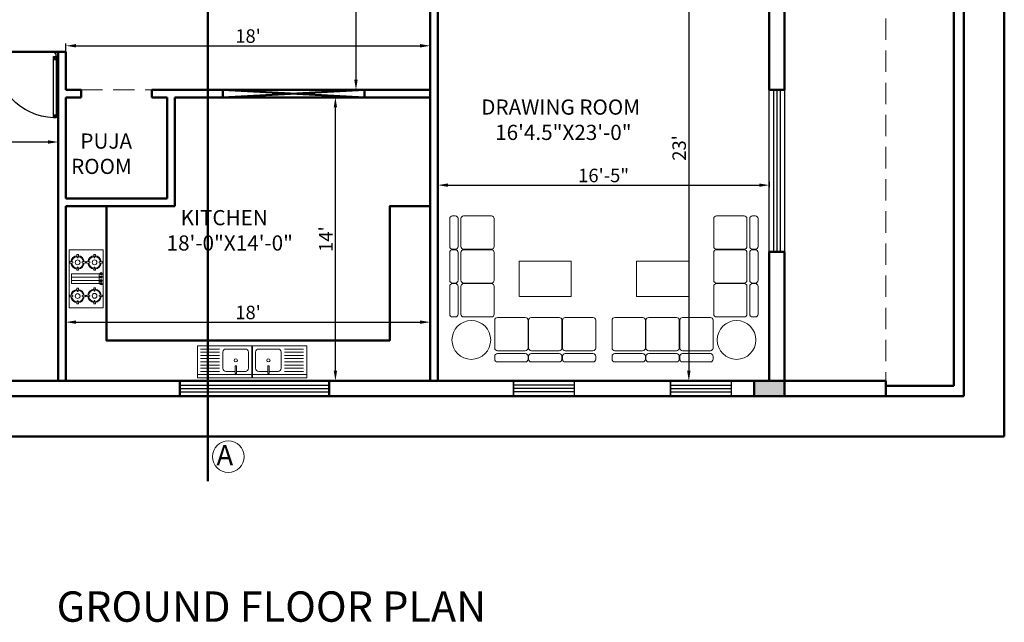
# Model space of a CAD drawing. Units: millimetres. Extents: x 1706 to 5913, y 156 to 1716.
# Tile 16 of 26: x 3489 to 4073, y 1031 to 1388. Entities that reach past the tile are written whole.
import ezdxf

# ---------------------------------------------------------------- set-up
doc = ezdxf.new("R2010")
doc.units = ezdxf.units.MM
doc.linetypes.add('DASHED', pattern=[19.05, 12.7, -6.35])
for name, color, linetype, lineweight in [('A-ANNO-DIMS', 2, 'Continuous', 18), ('A-ANNO-SYMB', 3, 'Continuous', 18), ('A-ANNO-TEXT', 7, 'Continuous', 18), ('A-AREA-IDEN', 3, 'Continuous', 18), ('A-COLS', 20, 'Continuous', 50), ('A-DOOR', 4, 'Continuous', 25), ('A-FLOR-OVHD', 9, 'DASHED', 18), ('A-FURN', 8, 'Continuous', 18), ('A-GLAZ', 150, 'Continuous', 25), ('A-WALL', 7, 'Continuous', 50)]:
    doc.layers.add(name, color=color, linetype=linetype, lineweight=lineweight)
doc.styles.get("Standard").update_dxf_attribs({"font": 'arial.ttf'})
doc.dimstyles.new('ISO-25', dxfattribs={"dimtxt": 8, "dimasz": 6, "dimexe": 1.25, "dimexo": 0.625, "dimtad": 1, "dimdec": 0, "dimlunit": 3, "dimtxsty": 'Standard', "dimcen": 2.5, "dimadec": 0, "dimazin": 0, "dimtfac": 1, "dimtdec": 0, "dimtmove": 0, "dimatfit": 3, "dimfxl": 1, "dimarcsym": 0})

# ---------------------------------------------------------------- blocks, each defined once
blk = doc.blocks.new('Puerta 01')
for p, q in [((-0.775, -0.026), (-0.737, -0.058)), ((-0.775, -0.058), (-0.737, -0.026)), ((-0.737, -0.058), (-0.737, -0.026)), ((-0.028, -0.058), (-0.066, -0.026)), ((-0.028, -0.026), (-0.066, -0.058)), ((-0.066, -0.058), (-0.066, -0.026))]:
    blk.add_line(p, q)
for points in [[(-0.028, 0), (-0.028, -0.026), (0.004, -0.026), (0.004, -0.036), (0.028, -0.036), (0.028, 0)], [(-0.028, -0.026), (-0.775, -0.026), (-0.775, -0.058), (-0.028, -0.058)], [(0.004, -0.774), (0.004, -0.764), (0.028, -0.764), (0.028, -0.8), (-0.028, -0.8), (-0.028, -0.774)]]:
    blk.add_lwpolyline(points, close=True)
blk.add_arc((-0.028, -0.026), 0.747, 182.4545, 270)
blk = doc.blocks.new('A$C57CF26DA')
for p, q in [((0, 0), (0, 420)), ((720, 420), (0, 420)), ((167, 413), (147, 413)), ((147, 413), (152, 373)), ((152, 373), (162, 373)), ((162, 373), (167, 413)), ((300, 391), (300, 49)), ((300, 391), (420, 391)), ((340, 391), (340, 49)), ((380, 391), (380, 49)), ((420, 391), (420, 49)), ((584, 413), (564, 413)), ((564, 413), (569, 373)), ((569, 373), (579, 373)), ((579, 373), (584, 413)), ((720, 0), (720, 420)), ((99, 320), (59, 325)), ((59, 325), (59, 305)), ((59, 305), (99, 310)), ((99, 310), (99, 320)), ((152, 257), (147, 217)), ((162, 257), (152, 257)), ((167, 217), (162, 257)), ((255, 325), (215, 320)), ((215, 320), (215, 310)), ((215, 310), (255, 305)), ((255, 305), (255, 325)), ((516, 320), (476, 325)), ((476, 325), (476, 305)), ((476, 305), (516, 310)), ((516, 310), (516, 320)), ((569, 257), (564, 217)), ((579, 257), (569, 257)), ((584, 217), (579, 257)), ((672, 325), (632, 320)), ((632, 320), (632, 310)), ((632, 310), (672, 305)), ((672, 305), (672, 325)), ((147, 217), (167, 217)), ((167, 203), (147, 203)), ((147, 203), (152, 163)), ((152, 163), (162, 163)), ((162, 163), (167, 203)), ((581, 203), (561, 203)), ((561, 203), (566, 163)), ((564, 217), (584, 217)), ((566, 163), (576, 163)), ((576, 163), (581, 203)), ((99, 110), (59, 115)), ((59, 115), (59, 95)), ((59, 95), (99, 100)), ((99, 100), (99, 110)), ((152, 47), (147, 7)), ((147, 7), (167, 7)), ((162, 47), (152, 47)), ((167, 7), (162, 47)), ((255, 115), (215, 110)), ((215, 110), (215, 100)), ((215, 100), (255, 95)), ((255, 95), (255, 115)), ((302, 39), (295, 39)), ((295, 39), (295, 11)), ((295, 11), (302, 11)), ((420, 49), (300, 49)), ((302, 11), (302, 39)), ((341, 39), (334, 39)), ((334, 39), (334, 11)), ((334, 11), (341, 11)), ((341, 11), (341, 39)), ((380, 11), (380, 39)), ((380, 39), (386, 39)), ((386, 11), (380, 11)), ((386, 39), (386, 11)), ((419, 11), (419, 39)), ((419, 39), (426, 39)), ((426, 11), (419, 11)), ((426, 39), (426, 11)), ((513, 110), (473, 115)), ((473, 115), (473, 95)), ((473, 95), (513, 100)), ((513, 100), (513, 110)), ((566, 47), (561, 7)), ((561, 7), (581, 7)), ((576, 47), (566, 47)), ((581, 7), (576, 47)), ((669, 115), (629, 110)), ((629, 110), (629, 100)), ((629, 100), (669, 95)), ((669, 95), (669, 115)), ((720, 0), (0, 0))]:
    blk.add_line(p, q)
for centre in [(157, 315), (574, 315), (157, 105), (571, 105)]:
    blk.add_circle(centre, 30)
for centre, radius, start, end in [((157, 315), 83, 95.5849, 174.4151), ((157, 315), 73, 95.3738, 174.6262), ((157, 315), 73, 5.3738, 84.6262), ((157, 315), 83, 5.5849, 84.4151), ((574, 315), 83, 95.5849, 174.4151), ((574, 315), 73, 95.3738, 174.6262), ((574, 315), 73, 5.3738, 84.6262), ((574, 315), 83, 5.5849, 84.4151), ((157, 315), 83, 185.5849, 264.4151), ((157, 315), 73, 185.3738, 264.6262), ((157, 315), 73, 275.3738, 354.6262), ((157, 315), 83, 275.5849, 354.4151), ((574, 315), 83, 185.5849, 264.4151), ((574, 315), 73, 185.3738, 264.6262), ((574, 315), 73, 275.3738, 354.6262), ((574, 315), 83, 275.5849, 354.4151), ((157, 105), 83, 95.5849, 174.4151), ((157, 105), 73, 95.3738, 174.6262), ((157, 105), 73, 5.3738, 84.6262), ((157, 105), 83, 5.5849, 84.4151), ((571, 105), 83, 95.5849, 174.4151), ((571, 105), 73, 95.3738, 174.6262), ((571, 105), 73, 5.3738, 84.6262), ((571, 105), 83, 5.5849, 84.4151), ((157, 105), 83, 185.5849, 264.4151), ((157, 105), 73, 185.3738, 264.6262), ((157, 105), 73, 275.3738, 354.6262), ((157, 105), 83, 275.5849, 354.4151), ((298, 25), 13.7, 104.4775, 255.5225), ((298, 25), 13.7, 284.4775, 75.5225), ((337, 25), 13.7, 104.4775, 255.5225), ((337, 25), 13.7, 284.4775, 75.5225), ((383, 25), 13.7, 104.4775, 255.5225), ((383, 25), 13.7, 284.4775, 75.5225), ((422, 25), 13.7, 104.4775, 255.5225), ((422, 25), 13.7, 284.4775, 75.5225), ((571, 105), 83, 185.5849, 264.4151), ((571, 105), 73, 185.3738, 264.6262), ((571, 105), 73, 275.3738, 354.6262), ((571, 105), 83, 275.5849, 354.4151)]:
    blk.add_arc(centre, radius, start, end)
blk = doc.blocks.new('A$C3404121D')
for p, q in [((0, 0), (0, 500)), ((0, 500), (850, 500)), ((850, 500), (850, 0)), ((0, 450), (850, 450)), ((50, 100), (50, 350)), ((100, 400), (240, 400)), ((240, 431), (240, 425)), ((260, 431), (240, 431)), ((240, 425), (240, 315)), ((240, 315), (260, 315)), ((260, 431), (260, 315)), ((260, 400), (400, 400)), ((450, 100), (450, 350)), ((502, 400), (801, 400)), ((502, 350), (801, 350)), ((502, 300), (801, 300)), ((502, 250), (801, 250)), ((502, 200), (801, 200)), ((850, 0), (0, 0)), ((400, 50), (100, 50)), ((502, 150), (801, 150)), ((502, 100), (801, 100)), ((801, 50), (502, 50))]:
    blk.add_line(p, q)
blk.add_circle((250, 228), 25)
for centre, start, end in [((100, 350), 90, 180), ((400, 350), 0, 90), ((100, 100), 180, 270), ((400, 100), 270, 0)]:
    blk.add_arc(centre, 50, start, end)
blk = doc.blocks.new('A$C753D6792')
at = {"linetype": 'ByBlock'}
for p, q in [((0, 2530), (0, 2580)), ((50, 2630), (550, 2630)), ((600, 2580), (600, 2530)), ((610, 2530), (610, 2580)), ((660, 2630), (1160, 2630)), ((1210, 2580), (1210, 2530)), ((1220, 2530), (1220, 2580)), ((1270, 2630), (1770, 2630)), ((1820, 2580), (1820, 2530)), ((0, 1880), (0, 2380)), ((550, 2480), (50, 2480)), ((550, 2430), (50, 2430)), ((600, 2380), (600, 1880)), ((610, 1880), (610, 2380)), ((1160, 2480), (660, 2480)), ((1160, 2430), (660, 2430)), ((1210, 2380), (1210, 1880)), ((1220, 1880), (1220, 2380)), ((1770, 2480), (1270, 2480)), ((1770, 2430), (1270, 2430)), ((1820, 1880), (1820, 2380)), ((50, 1830), (427, 1830)), ((387, 1830), (550, 1830)), ((660, 1830), (1037, 1830)), ((997, 1830), (1160, 1830)), ((1270, 1830), (1647, 1830)), ((1607, 1830), (1770, 1830)), ((1880, 1820), (2380, 1820)), ((2530, 1820), (2580, 1820)), ((1830, 1770), (1830, 1393)), ((2430, 1270), (2430, 1770)), ((2480, 1270), (2480, 1770)), ((2630, 1770), (2630, 1270)), ((442, 815), (442, 1455)), ((442, 1455), (1372, 1455)), ((1382, 1455), (1382, 815)), ((1830, 1433), (1830, 1270)), ((1830, 1160), (1830, 783)), ((2380, 1220), (1880, 1220)), ((1880, 1210), (2380, 1210)), ((2430, 660), (2430, 1160)), ((2480, 660), (2480, 1160)), ((2580, 1220), (2530, 1220)), ((2530, 1210), (2580, 1210)), ((2630, 1160), (2630, 660)), ((1382, 815), (442, 815)), ((1830, 823), (1830, 660)), ((1830, 550), (1830, 173)), ((2380, 610), (1880, 610)), ((1880, 600), (2380, 600)), ((2430, 50), (2430, 550)), ((2480, 50), (2480, 550)), ((2580, 610), (2530, 610)), ((2530, 600), (2580, 600)), ((2630, 550), (2630, 50)), ((1830, 213), (1830, 50)), ((2380, 0), (1880, 0)), ((2580, 0), (2530, 0))]:
    blk.add_line(p, q, dxfattribs=at)
blk.add_circle((2242, 2235), 349, dxfattribs=at)
for centre, start, end in [((50, 2580), 90, 180), ((50, 2530), 180, 270), ((550, 2580), 0, 90), ((550, 2580), 0, 90), ((550, 2530), 270, 0), ((550, 2530), 270, 0), ((660, 2580), 90, 180), ((660, 2530), 180, 270), ((1160, 2580), 0, 90), ((1160, 2580), 0, 90), ((1160, 2530), 270, 0), ((1160, 2530), 270, 0), ((1270, 2580), 90, 180), ((1270, 2530), 180, 270), ((1770, 2580), 0, 90), ((1770, 2580), 0, 90), ((1770, 2530), 270, 0), ((1770, 2530), 270, 0), ((50, 2380), 90, 180), ((550, 2380), 0, 90), ((550, 2380), 0, 90), ((660, 2380), 90, 180), ((1160, 2380), 0, 90), ((1160, 2380), 0, 90), ((1270, 2380), 90, 180), ((1770, 2380), 0, 90), ((1770, 2380), 0, 90), ((50, 1880), 180, 270), ((550, 1880), 270, 0), ((660, 1880), 180, 270), ((1160, 1880), 270, 0), ((1270, 1880), 180, 270), ((1770, 1880), 270, 0), ((1880, 1770), 90, 180), ((2380, 1770), 0, 90), ((2530, 1770), 90, 180), ((2580, 1770), 0, 90), ((1880, 1270), 180, 270), ((2380, 1270), 270, 0), ((2380, 1270), 270, 0), ((2530, 1270), 180, 270), ((2530, 1270), 180, 270), ((2580, 1270), 270, 0), ((2580, 1270), 270, 0), ((1880, 1160), 90, 180), ((2380, 1160), 0, 90), ((2530, 1160), 90, 180), ((2580, 1160), 0, 90), ((1880, 660), 180, 270), ((1880, 550), 90, 180), ((2380, 660), 270, 0), ((2380, 660), 270, 0), ((2380, 550), 0, 90), ((2530, 660), 180, 270), ((2530, 660), 180, 270), ((2530, 550), 90, 180), ((2580, 660), 270, 0), ((2580, 660), 270, 0), ((2580, 550), 0, 90), ((1880, 50), 180, 270), ((2380, 50), 270, 0), ((2380, 50), 270, 0), ((2530, 50), 180, 270), ((2530, 50), 180, 270), ((2580, 50), 270, 0), ((2580, 50), 270, 0)]:
    blk.add_arc(centre, 50, start, end, dxfattribs=at)
blk = doc.blocks.new('*D51')
at = {"layer": 'A-ANNO-DIMS', "color": 0, "lineweight": -2, "transparency": 16777216}
for p, q in [((3231.71, 1314.9), (3231.71, 1316.48)), ((3237.71, 1315.23), (3506.21, 1315.23)), ((3512.21, 1314.9), (3512.21, 1316.48))]:
    blk.add_line(p, q, dxfattribs=at)
at = {"layer": 'A-ANNO-DIMS', "color": 0, "transparency": 16777216}
for points in [[(3237.71, 1316.23), (3237.71, 1314.23), (3231.71, 1315.23)], [(3506.21, 1316.23), (3506.21, 1314.23), (3512.21, 1315.23)]]:
    blk.add_solid(points, dxfattribs=at)
at = {"layer": 'Defpoints', "color": 0, "transparency": 16777216}
for p in [(3231.71, 1314.27), (3512.21, 1315.23), (3512.21, 1314.27)]:
    blk.add_point(p, dxfattribs=at)
at = {"layer": 'A-ANNO-DIMS', "color": 0, "transparency": 16777216, "insert": (3371.96, 1319.94), "char_height": 8, "attachment_point": 5}
blk.add_mtext('23\'-5"', dxfattribs=at)
blk = doc.blocks.new('*D58')
at = {"layer": 'A-ANNO-DIMS', "color": 0, "lineweight": -2, "transparency": 16777216}
for p, q in [((3686.08, 1503.68), (3689.93, 1503.68)), ((3688.68, 1497.68), (3688.68, 1352.18)), ((3686.08, 1346.18), (3689.93, 1346.18))]:
    blk.add_line(p, q, dxfattribs=at)
at = {"layer": 'A-ANNO-DIMS', "color": 0, "transparency": 16777216}
for points in [[(3687.68, 1497.68), (3689.68, 1497.68), (3688.68, 1503.68)], [(3687.68, 1352.18), (3689.68, 1352.18), (3688.68, 1346.18)]]:
    blk.add_solid(points, dxfattribs=at)
at = {"layer": 'Defpoints', "color": 0, "transparency": 16777216}
for p in [(3685.46, 1503.68), (3685.46, 1346.18), (3688.68, 1346.18)]:
    blk.add_point(p, dxfattribs=at)
at = {"layer": 'A-ANNO-DIMS', "color": 0, "transparency": 16777216, "insert": (3683.97, 1424.93), "char_height": 8, "attachment_point": 5, "rotation": 90}
blk.add_mtext('13\'-2"', dxfattribs=at)
blk = doc.blocks.new('*D59')
at = {"layer": 'A-ANNO-DIMS', "color": 0, "lineweight": -2, "transparency": 16777216}
for p, q in [((3516.71, 1359.93), (3516.71, 1373.5)), ((3522.71, 1372.25), (3726.71, 1372.25)), ((3732.71, 1359.93), (3732.71, 1373.5))]:
    blk.add_line(p, q, dxfattribs=at)
at = {"layer": 'A-ANNO-DIMS', "color": 0, "transparency": 16777216}
for points in [[(3522.71, 1373.25), (3522.71, 1371.25), (3516.71, 1372.25)], [(3726.71, 1373.25), (3726.71, 1371.25), (3732.71, 1372.25)]]:
    blk.add_solid(points, dxfattribs=at)
at = {"layer": 'Defpoints', "color": 0, "transparency": 16777216}
for p in [(3732.71, 1372.25), (3516.71, 1359.3), (3732.71, 1359.3)]:
    blk.add_point(p, dxfattribs=at)
at = {"layer": 'A-ANNO-DIMS', "color": 0, "transparency": 16777216, "insert": (3624.71, 1376.96), "char_height": 8, "attachment_point": 5}
blk.add_mtext("18'", dxfattribs=at)
blk = doc.blocks.new('*D60')
at = {"layer": 'A-ANNO-DIMS', "color": 0, "lineweight": -2, "transparency": 16777216}
for p, q in [((3677.47, 1341.68), (3675.23, 1341.68)), ((3676.48, 1179.68), (3676.48, 1335.68)), ((3677.47, 1173.68), (3675.23, 1173.68))]:
    blk.add_line(p, q, dxfattribs=at)
at = {"layer": 'A-ANNO-DIMS', "color": 0, "transparency": 16777216}
for points in [[(3675.48, 1335.68), (3677.48, 1335.68), (3676.48, 1341.68)], [(3675.48, 1179.68), (3677.48, 1179.68), (3676.48, 1173.68)]]:
    blk.add_solid(points, dxfattribs=at)
at = {"layer": 'Defpoints', "color": 0, "transparency": 16777216}
for p in [(3676.48, 1341.68), (3678.09, 1341.68), (3678.09, 1173.68)]:
    blk.add_point(p, dxfattribs=at)
at = {"layer": 'A-ANNO-DIMS', "color": 0, "transparency": 16777216, "insert": (3671.84, 1257.68), "char_height": 8, "attachment_point": 5, "rotation": 90}
blk.add_mtext("14'", dxfattribs=at)
blk = doc.blocks.new('*D61')
at = {"layer": 'A-ANNO-DIMS', "color": 0, "lineweight": -2, "transparency": 16777216}
for p, q in [((3516.71, 1201.14), (3516.71, 1209.73)), ((3522.71, 1208.48), (3726.71, 1208.48)), ((3732.71, 1201.14), (3732.71, 1209.73))]:
    blk.add_line(p, q, dxfattribs=at)
at = {"layer": 'A-ANNO-DIMS', "color": 0, "transparency": 16777216}
for points in [[(3522.71, 1209.48), (3522.71, 1207.48), (3516.71, 1208.48)], [(3726.71, 1209.48), (3726.71, 1207.48), (3732.71, 1208.48)]]:
    blk.add_solid(points, dxfattribs=at)
at = {"layer": 'Defpoints', "color": 0, "transparency": 16777216}
for p in [(3732.71, 1208.48), (3516.71, 1200.51), (3732.71, 1200.51)]:
    blk.add_point(p, dxfattribs=at)
at = {"layer": 'A-ANNO-DIMS', "color": 0, "transparency": 16777216, "insert": (3624.71, 1213.19), "char_height": 8, "attachment_point": 5}
blk.add_mtext("18'", dxfattribs=at)
blk = doc.blocks.new('*D62')
at = {"layer": 'A-ANNO-DIMS', "color": 0, "lineweight": -2, "transparency": 16777216}
for p, q in [((3882.51, 1449.68), (3887.24, 1449.68)), ((3885.99, 1443.68), (3885.99, 1179.68)), ((3882.51, 1173.68), (3887.24, 1173.68))]:
    blk.add_line(p, q, dxfattribs=at)
at = {"layer": 'A-ANNO-DIMS', "color": 0, "transparency": 16777216}
for points in [[(3884.99, 1443.68), (3886.99, 1443.68), (3885.99, 1449.68)], [(3884.99, 1179.68), (3886.99, 1179.68), (3885.99, 1173.68)]]:
    blk.add_solid(points, dxfattribs=at)
at = {"layer": 'Defpoints', "color": 0, "transparency": 16777216}
for p in [(3881.89, 1449.68), (3881.89, 1173.68), (3885.99, 1173.68)]:
    blk.add_point(p, dxfattribs=at)
at = {"layer": 'A-ANNO-DIMS', "color": 0, "transparency": 16777216, "insert": (3881.28, 1311.68), "char_height": 8, "attachment_point": 5, "rotation": 90}
blk.add_mtext("23'", dxfattribs=at)
blk = doc.blocks.new('*D63')
at = {"layer": 'A-ANNO-DIMS', "color": 0, "lineweight": -2, "transparency": 16777216}
for p, q in [((3737.21, 1291.56), (3737.21, 1288.41)), ((3933.71, 1291.56), (3933.71, 1288.41)), ((3743.21, 1289.66), (3927.71, 1289.66))]:
    blk.add_line(p, q, dxfattribs=at)
at = {"layer": 'A-ANNO-DIMS', "color": 0, "transparency": 16777216}
for points in [[(3743.21, 1290.66), (3743.21, 1288.66), (3737.21, 1289.66)], [(3927.71, 1290.66), (3927.71, 1288.66), (3933.71, 1289.66)]]:
    blk.add_solid(points, dxfattribs=at)
at = {"layer": 'Defpoints', "color": 0, "transparency": 16777216}
for p in [(3737.21, 1292.18), (3933.71, 1292.18), (3933.71, 1289.66)]:
    blk.add_point(p, dxfattribs=at)
at = {"layer": 'A-ANNO-DIMS', "color": 0, "transparency": 16777216, "insert": (3835.46, 1294.37), "char_height": 8, "attachment_point": 5}
blk.add_mtext('16\'-5"', dxfattribs=at)

msp = doc.modelspace()

# ---------------------------------------------------------------- hatches: boundary and pattern name
at = {"layer": 'A-COLS'}
h = msp.add_hatch(color=256, dxfattribs=at)
h.dxf.hatch_style = 1
h.paths.add_polyline_path([(3942.71, 1173.68), (3924.71, 1173.68), (3924.71, 1164.68), (3942.71, 1164.68)])

# ---------------------------------------------------------------- linework, layer by layer
at = {"layer": 'A-ANNO-SYMB'}
msp.add_circle((3613.03, 1128.74), 9.38, dxfattribs=at)
at = {"layer": 'A-COLS'}
msp.add_lwpolyline([(3942.93, 1173.68), (3924.71, 1173.68), (3924.71, 1164.68), (3942.71, 1164.68), (3942.71, 1173.68)], dxfattribs=at)
at = {"layer": 'A-FLOR-OVHD'}
for p, q in [((4002.71, 1655.18), (4002.71, 1173.68)), ((3525.71, 1346.18), (3567.71, 1346.18))]:
    msp.add_line(p, q, dxfattribs=at)
at = {"layer": 'A-GLAZ'}
for p, q in [((3936.21, 1346.18), (3936.21, 1250.18)), ((3938.21, 1346.18), (3938.21, 1250.18)), ((3940.21, 1346.18), (3940.21, 1250.18)), ((3782.07, 1173.68), (3782.07, 1164.68)), ((3818.07, 1173.68), (3818.07, 1164.68)), ((3875.07, 1173.68), (3875.07, 1164.68)), ((3911.07, 1173.68), (3911.07, 1164.68)), ((3584.21, 1171.18), (3672.71, 1171.18)), ((3584.21, 1169.18), (3672.71, 1169.18)), ((3818.07, 1171.18), (3782.07, 1171.18)), ((3818.07, 1169.18), (3782.07, 1169.18)), ((3875.07, 1171.18), (3911.07, 1171.18)), ((3875.07, 1169.18), (3911.07, 1169.18)), ((3584.21, 1167.18), (3672.71, 1167.18)), ((3818.07, 1167.18), (3782.07, 1167.18)), ((3875.07, 1167.18), (3911.07, 1167.18))]:
    msp.add_line(p, q, dxfattribs=at)
for points in [[(3933.71, 1346.18), (3942.71, 1346.18), (3942.71, 1250.18), (3933.71, 1250.18)], [(3584.21, 1173.68), (3672.71, 1173.68), (3672.71, 1164.68), (3584.21, 1164.68)], [(3782.07, 1173.68), (3818.07, 1173.68), (3818.07, 1164.68), (3782.07, 1164.68)], [(3875.07, 1173.68), (3911.07, 1173.68), (3911.07, 1164.68), (3875.07, 1164.68)]]:
    msp.add_lwpolyline(points, close=True, dxfattribs=at)
at = {"layer": 'A-WALL'}
for p, q in [((3600.83, 1703), (3600.83, 1114.32)), ((4049, 1664.18), (4049, 1164.68)), ((4073, 1664.18), (4073, 1140.68)), ((4043, 1658.18), (4043, 1170.68)), ((3732.71, 1410.68), (3732.71, 1173.68)), ((3737.21, 1410.68), (3737.21, 1173.68)), ((3933.71, 1403.18), (3933.71, 1346.18)), ((3942.71, 1403.18), (3942.71, 1346.18)), ((3473.21, 1368.68), (3512.21, 1368.68)), ((3512.21, 1368.68), (3516.71, 1368.68)), ((3512.21, 1368.68), (3512.21, 1173.68)), ((3516.71, 1368.68), (3516.71, 1346.18)), ((3516.71, 1346.18), (3525.71, 1346.18)), ((3525.71, 1346.18), (3525.71, 1341.68)), ((3567.71, 1346.18), (3567.71, 1341.68)), ((3567.71, 1346.18), (3609.71, 1346.18)), ((3609.71, 1346.18), (3609.71, 1341.68)), ((3693.71, 1346.18), (3609.71, 1341.68)), ((3609.71, 1346.18), (3693.71, 1341.68)), ((3693.71, 1346.18), (3693.71, 1341.68)), ((3693.71, 1346.18), (3732.71, 1346.18)), ((3942.71, 1346.18), (3933.71, 1346.18)), ((3516.71, 1341.68), (3525.71, 1341.68)), ((3516.71, 1341.68), (3516.71, 1281.68)), ((3567.71, 1341.68), (3576.71, 1341.68)), ((3576.71, 1341.68), (3576.71, 1281.68)), ((3581.21, 1341.68), (3581.21, 1277.18)), ((3581.21, 1341.68), (3609.71, 1341.68)), ((3693.71, 1341.68), (3732.71, 1341.68)), ((3516.71, 1281.68), (3576.71, 1281.68)), ((3516.71, 1277.18), (3581.21, 1277.18)), ((3516.71, 1277.18), (3516.71, 1173.68)), ((3942.71, 1250.18), (3933.71, 1250.18)), ((3933.71, 1250.18), (3933.71, 1173.68)), ((3942.71, 1250.18), (3942.71, 1173.68)), ((3207.71, 1173.68), (4002.71, 1173.68)), ((3584.21, 1173.68), (3584.21, 1164.68)), ((3672.71, 1173.68), (3672.71, 1164.68)), ((3942.71, 1173.68), (3942.71, 1164.68)), ((3942.71, 1164.68), (3942.71, 1173.68)), ((4002.71, 1173.68), (4002.71, 1164.68)), ((4043, 1170.68), (4002.71, 1170.68)), ((3203.21, 1164.68), (4002.71, 1164.68)), ((4049, 1164.68), (4002.71, 1164.68)), ((3177.71, 1140.68), (4073, 1140.68))]:
    msp.add_line(p, q, dxfattribs=at)
msp.add_lwpolyline([(3609.71, 1346.18), (3693.71, 1346.18), (3693.71, 1341.68), (3609.71, 1341.68)], close=True, dxfattribs=at)
msp.add_lwpolyline([(3540.71, 1277.18), (3540.71, 1197.68), (3708.71, 1197.68), (3708.71, 1277.18), (3732.71, 1277.18)], dxfattribs=at)

# ---------------------------------------------------------------- block references
at = {"layer": 'A-DOOR', "extrusion": (0, 0, -1), "xscale": 48.75000000000294, "yscale": 48.75000000000294, "zscale": -48.75000000000287, "rotation": 89.99999999879581}
msp.add_blockref('Puerta 01', (-3512.21, 1367.32), dxfattribs=at)
at = {"layer": 'A-FURN'}
for name, p, xscale, yscale, zscale, rotation in [('A$C753D6792', (3830.82, 1271.46), 0.0329035460231199, 0.0329035460231199, 0.0329035460231199, 180), ('A$C753D6792', (3840.51, 1271.46), -0.0329035460231199, 0.0329035460231199, 0.0329035460231199, 180), ('A$C57CF26DA', (3538.75, 1251.41), -0.0478777176975714, 0.0478777176975714, 0.0478777176975714, 90), ('A$C3404121D', (3626.89, 1194.45), 0.0378984485580132, 0.0378984485580132, 0.0378984485580132, 180), ('A$C3404121D', (3627.3, 1194.45), -0.0378984485580132, 0.0378984485580132, 0.0378984485580132, 180)]:
    msp.add_blockref(name, p, dxfattribs=dict(at, xscale=xscale, yscale=yscale, zscale=zscale, rotation=rotation))

# ---------------------------------------------------------------- texts
at = {"layer": 'A-ANNO-SYMB', "insert": (3602.29, 1135.61), "char_height": 12, "attachment_point": 1}
msp.add_mtext_dynamic_manual_height_columns(' A', width=23.3743, gutter_width=12.5, heights=[0], dxfattribs=at)
at = {"layer": 'A-ANNO-TEXT', "insert": (3511.24, 1048.93), "char_height": 18, "attachment_point": 1}
msp.add_mtext_dynamic_manual_height_columns('GROUND FLOOR PLAN', width=352.5721, gutter_width=12.5, heights=[0], dxfattribs=at)
at = {"layer": 'A-AREA-IDEN', "char_height": 9, "attachment_point": 1}
for s, width, insert in [('    DRAWING ROOM\\P       16\'4.5"X23\'-0"', 125.2434, (3751.91, 1340.43)), ('  PUJA ROOM', 67.9131, (3519.8, 1320.28)), ('    KITCHEN\\P 18\'-0"X14\'-0"', 99.443, (3573.66, 1274.89))]:
    msp.add_mtext_dynamic_manual_height_columns(s, width=width, gutter_width=12.5, heights=[0], dxfattribs=dict(at, insert=insert))

# ---------------------------------------------------------------- dimensions: what is measured, and where the dimension line sits
at = {"layer": 'A-ANNO-DIMS'}
for base, p1, p2, picture, middle in [((3688.68200939, 1346.18004162), (3685.45687195, 1503.68004162), (3685.45687195, 1346.18004162), '*D58', (3683.96969697, 1424.93004162)), ((3885.99, 1173.68), (3881.89, 1449.68), (3881.89, 1173.68), '*D62', (3881.28, 1311.68)), ((3676.48, 1341.68), (3678.09, 1173.68), (3678.09, 1341.68), '*D60', (3671.84, 1257.68))]:
    dim = msp.add_linear_dim(base=base, p1=p1, p2=p2, angle=90, dimstyle='ISO-25', override={"dimclrd": 0, "dimclre": 0, "dimclrt": 0}, dxfattribs=at)
    dim.commit()
    dim.dimension.update_dxf_attribs({"geometry": picture, "text_midpoint": middle})
for base, p1, p2, picture, middle in [((3732.71, 1372.25), (3516.71, 1359.3), (3732.71, 1359.3), '*D59', (3624.71, 1376.96)), ((3512.20687195, 1315.2255673), (3231.70687195, 1314.27053736), (3512.20687195, 1314.27053736), '*D51', (3371.95687195, 1319.93787971)), ((3933.70687195, 1289.66249214), (3737.20687195, 1292.18004162), (3933.70687195, 1292.18004162), '*D63', (3835.45687195, 1294.37207604)), ((3732.71, 1208.48), (3516.71, 1200.51), (3732.71, 1200.51), '*D61', (3624.71, 1213.19))]:
    dim = msp.add_linear_dim(base=base, p1=p1, p2=p2, dimstyle='ISO-25', override={"dimclrd": 0, "dimclre": 0, "dimclrt": 0}, dxfattribs=at)
    dim.commit()
    dim.dimension.update_dxf_attribs({"geometry": picture, "text_midpoint": middle})

doc.saveas('drawing.dxf')
